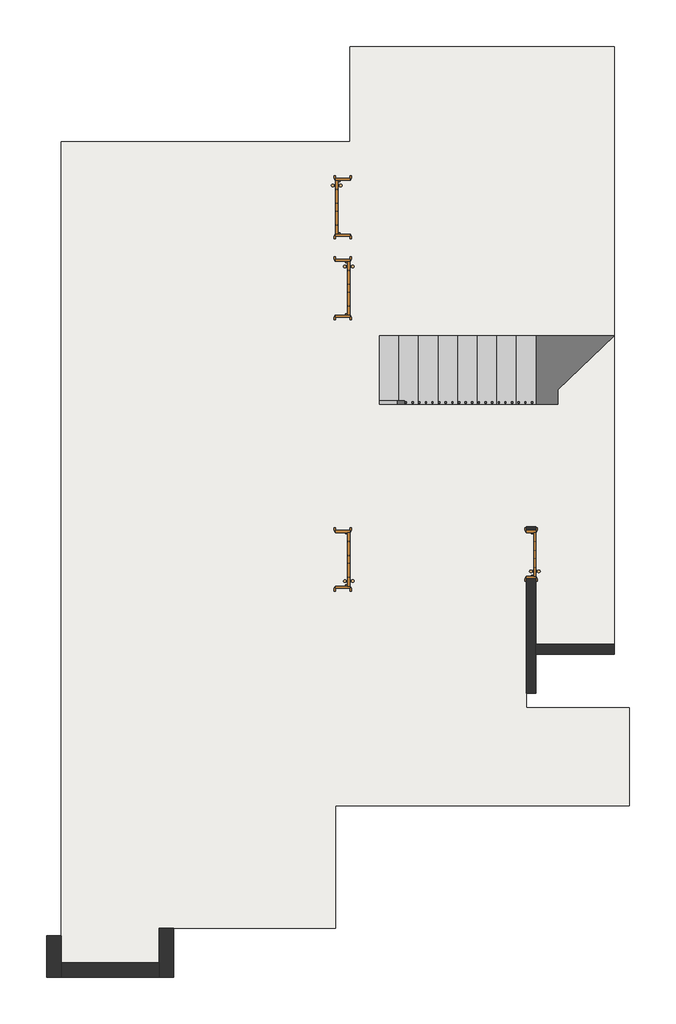
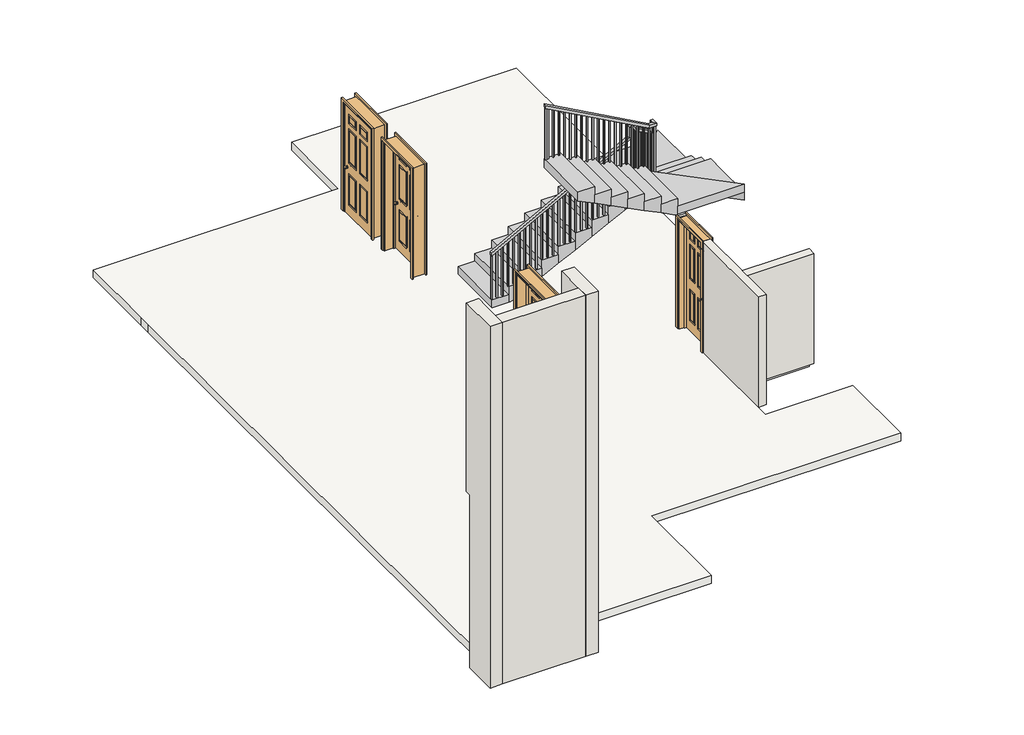
# One storey: 5 walls, 4 doors, 1 railing, 1 slab, 1 stair flight.
"""IFC4 building model written with IfcOpenShell, lengths in millimetres."""

from ifc_helpers import new_model, si_unit, frame, origin, place, context, project, spatial, polyline, outline, extrude, faceted_brep, transform, mapped, element, save
from components import intsgl_9_d1_c400c9dc, intsgl_9_d1_bc548916, intsgl_9_d2_a593ccd7

model = new_model("IFC4")

# Units and contexts
model_context = context("Model", 3, world=origin())
ifc_project = project(units=[si_unit("LENGTHUNIT", "METRE", prefix="MILLI")], contexts=[model_context])

# Site, building, storey
site = spatial("IfcSite", under=ifc_project)
building = spatial("IfcBuilding", under=site)
storey = spatial("IfcBuildingStorey", under=building, Elevation=600.0)

# Doors
placement = place(None, origin())
intsgl_9_d1_shape = intsgl_9_d1_c400c9dc(model_context)
element("IfcDoor", 1, ObjectType="IntSgl (9) : D1", at=placement, inside=storey, context=model_context, shape_type="MappedRepresentation", body=[
    mapped(intsgl_9_d1_shape, transform((-10030.1792561, 3948.2802318, 600.0), x_axis=(0.0, -1.0, 0.0), y_axis=(1.0, 0.0, 0.0), z_axis=(0.0, 0.0, 1.0))),
])
intsgl_9_d1_2_shape = intsgl_9_d1_bc548916(model_context)
element("IfcDoor", 2, ObjectType="IntSgl (9) : D1", at=placement, inside=storey, context=model_context, shape_type="MappedRepresentation", body=[
    mapped(intsgl_9_d1_2_shape, transform((-10030.1792561, 5188.2802318, 600.0), x_axis=(0.0, -1.0, 0.0), y_axis=(1.0, 0.0, 0.0), z_axis=(0.0, 0.0, 1.0))),
])
element("IfcDoor", 3, ObjectType="IntSgl (9) : D1", at=placement, inside=storey, context=model_context, shape_type="MappedRepresentation", body=[
    mapped(intsgl_9_d1_2_shape, transform((-10030.1792561, -201.7197682, 600.0), x_axis=(0.0, 1.0, 0.0), y_axis=(-1.0, 0.0, 0.0), z_axis=(0.0, 0.0, 1.0))),
])
intsgl_9_d2_shape = intsgl_9_d2_a593ccd7(model_context)
element("IfcDoor", 4, ObjectType="IntSgl (9) : D2", at=placement, inside=storey, context=model_context, shape_type="MappedRepresentation", body=[
    mapped(intsgl_9_d2_shape, transform((-7142.6792561, -126.7197682, 600.0), x_axis=(0.0, 1.0, 0.0), y_axis=(-1.0, 0.0, 0.0), z_axis=(0.0, 0.0, 1.0))),
])

# Railing
element("IfcRailing", 5, ObjectType="Handrail - Rectangular", at=placement, inside=storey, context=model_context, shape_type="SolidModel", body=[
    faceted_brep([(-9467.6792561, 2223.6802318, 1650.0), (-9467.6792561, 2223.6802318, 1593.1757094), (-9467.6792561, 2173.6802318, 1593.1757094), (-9467.6792561, 2173.6802318, 1650.0), (-6992.2792561, 2223.6802318, 2986.716), (-6942.2792561, 2223.6802318, 2956.8917094), (-6942.2792561, 2173.6802318, 2956.8917094), (-6992.2792561, 2173.6802318, 2986.716), (-6992.2792561, 2223.6802318, 3187.3), (-6942.2792561, 2223.6802318, 3137.3), (-6942.2792561, 2173.6802318, 3137.3), (-6992.2792561, 2173.6802318, 3187.3), (-6867.2792561, 2223.6802318, 3187.3), (-6867.2792561, 2223.6802318, 3137.3), (-6917.2792561, 2173.6802318, 3137.3), (-6917.2792561, 2173.6802318, 3187.3), (-6867.2792561, 2098.6802318, 3187.3), (-6867.2792561, 2086.8768329, 3137.3), (-6917.2792561, 2086.8768329, 3137.3), (-6917.2792561, 2098.6802318, 3187.3), (-6867.2792561, 1647.8802318, 3412.7), (-6867.2792561, 1597.8802318, 3381.7983006), (-6917.2792561, 1597.8802318, 3381.7983006), (-6917.2792561, 1647.8802318, 3412.7), (-6867.2792561, 1647.8802318, 3613.5947368), (-6867.2792561, 1597.8802318, 3563.5947368), (-6917.2792561, 1597.8802318, 3563.5947368), (-6917.2792561, 1647.8802318, 3613.5947368), (-6867.2792561, 1522.8802318, 3613.5947368), (-6867.2792561, 1522.8802318, 3563.5947368), (-6917.2792561, 1572.8802318, 3563.5947368), (-6917.2792561, 1572.8802318, 3613.5947368), (-6992.2792561, 1522.8802318, 3613.5947368), (-7005.1758911, 1522.8802318, 3563.5947368), (-7005.1758911, 1572.8802318, 3563.5947368), (-6992.2792561, 1572.8802318, 3613.5947368), (-8867.6792561, 1522.8802318, 4650.0), (-8867.6792561, 1572.8802318, 4650.0), (-8867.6792561, 1572.8802318, 4592.8729122), (-8867.6792561, 1522.8802318, 4592.8729122)], [[[0, 1, 2, 3]], [[1, 0, 4, 5]], [[2, 1, 5, 6]], [[3, 2, 6, 7]], [[0, 3, 7, 4]], [[5, 4, 8, 9]], [[6, 5, 9, 10]], [[7, 6, 10, 11]], [[4, 7, 11, 8]], [[9, 8, 12, 13]], [[10, 9, 13, 14]], [[11, 10, 14, 15]], [[8, 11, 15, 12]], [[13, 12, 16, 17]], [[14, 13, 17, 18]], [[15, 14, 18, 19]], [[12, 15, 19, 16]], [[17, 16, 20, 21]], [[18, 17, 21, 22]], [[19, 18, 22, 23]], [[16, 19, 23, 20]], [[21, 20, 24, 25]], [[22, 21, 25, 26]], [[23, 22, 26, 27]], [[20, 23, 27, 24]], [[25, 24, 28, 29]], [[26, 25, 29, 30]], [[27, 26, 30, 31]], [[24, 27, 31, 28]], [[29, 28, 32, 33]], [[30, 29, 33, 34]], [[31, 30, 34, 35]], [[28, 31, 35, 32]], [[36, 37, 38, 39]], [[33, 32, 36, 39]], [[34, 33, 39, 38]], [[35, 34, 38, 37]], [[32, 35, 37, 36]]]),
    extrude(outline(polyline([(3600.0, -8812.6792561), (4562.4781754, -8812.6792561), (4573.530807, -8832.6792561), (3600.0, -8832.6792561), (3600.0, -8812.6792561)])), frame((0.0, 1537.8802318, 0.0), z_axis=(0.0, 1.0, 0.0), x_axis=(0.0, 0.0, 1.0)), (0.0, 0.0, 1.0), 20.0),
    extrude(outline(polyline([(3600.0, -8711.0792561), (4506.330807, -8711.0792561), (4517.3834386, -8731.0792561), (3600.0, -8731.0792561), (3600.0, -8711.0792561)])), frame((0.0, 1537.8802318, 0.0), z_axis=(0.0, 1.0, 0.0), x_axis=(0.0, 0.0, 1.0)), (0.0, 0.0, 1.0), 20.0),
    extrude(outline(polyline([(3600.0, -8609.4792561), (4450.1834386, -8609.4792561), (4461.2360701, -8629.4792561), (3600.0, -8629.4792561), (3600.0, -8609.4792561)])), frame((0.0, 1537.8802318, 0.0), z_axis=(0.0, 1.0, 0.0), x_axis=(0.0, 0.0, 1.0)), (0.0, 0.0, 1.0), 20.0),
    extrude(outline(polyline([(3450.0, -8507.8792561), (4394.0360701, -8507.8792561), (4405.0887017, -8527.8792561), (3450.0, -8527.8792561), (3450.0, -8507.8792561)])), frame((0.0, 1537.8802318, 0.0), z_axis=(0.0, 1.0, 0.0), x_axis=(0.0, 0.0, 1.0)), (0.0, 0.0, 1.0), 20.0),
    extrude(outline(polyline([(3450.0, -8406.2792561), (4337.8887017, -8406.2792561), (4348.9413333, -8426.2792561), (3450.0, -8426.2792561), (3450.0, -8406.2792561)])), frame((0.0, 1537.8802318, 0.0), z_axis=(0.0, 1.0, 0.0), x_axis=(0.0, 0.0, 1.0)), (0.0, 0.0, 1.0), 20.0),
    extrude(outline(polyline([(3450.0, -8304.6792561), (4281.7413333, -8304.6792561), (4292.7939649, -8324.6792561), (3450.0, -8324.6792561), (3450.0, -8304.6792561)])), frame((0.0, 1537.8802318, 0.0), z_axis=(0.0, 1.0, 0.0), x_axis=(0.0, 0.0, 1.0)), (0.0, 0.0, 1.0), 20.0),
    extrude(outline(polyline([(3300.0, -8203.0792561), (4225.5939649, -8203.0792561), (4236.6465965, -8223.0792561), (3300.0, -8223.0792561), (3300.0, -8203.0792561)])), frame((0.0, 1537.8802318, 0.0), z_axis=(0.0, 1.0, 0.0), x_axis=(0.0, 0.0, 1.0)), (0.0, 0.0, 1.0), 20.0),
    extrude(outline(polyline([(3300.0, -8101.4792561), (4169.4465965, -8101.4792561), (4180.499228, -8121.4792561), (3300.0, -8121.4792561), (3300.0, -8101.4792561)])), frame((0.0, 1537.8802318, 0.0), z_axis=(0.0, 1.0, 0.0), x_axis=(0.0, 0.0, 1.0)), (0.0, 0.0, 1.0), 20.0),
    extrude(outline(polyline([(3300.0, -7999.8792561), (4113.299228, -7999.8792561), (4124.3518596, -8019.8792561), (3300.0, -8019.8792561), (3300.0, -7999.8792561)])), frame((0.0, 1537.8802318, 0.0), z_axis=(0.0, 1.0, 0.0), x_axis=(0.0, 0.0, 1.0)), (0.0, 0.0, 1.0), 20.0),
    extrude(outline(polyline([(3150.0, -7898.2792561), (4057.1518596, -7898.2792561), (4068.2044912, -7918.2792561), (3150.0, -7918.2792561), (3150.0, -7898.2792561)])), frame((0.0, 1537.8802318, 0.0), z_axis=(0.0, 1.0, 0.0), x_axis=(0.0, 0.0, 1.0)), (0.0, 0.0, 1.0), 20.0),
    extrude(outline(polyline([(3150.0, -7796.6792561), (4001.0044912, -7796.6792561), (4012.0571228, -7816.6792561), (3150.0, -7816.6792561), (3150.0, -7796.6792561)])), frame((0.0, 1537.8802318, 0.0), z_axis=(0.0, 1.0, 0.0), x_axis=(0.0, 0.0, 1.0)), (0.0, 0.0, 1.0), 20.0),
    extrude(outline(polyline([(3150.0, -7695.0792561), (3944.8571228, -7695.0792561), (3955.9097544, -7715.0792561), (3150.0, -7715.0792561), (3150.0, -7695.0792561)])), frame((0.0, 1537.8802318, 0.0), z_axis=(0.0, 1.0, 0.0), x_axis=(0.0, 0.0, 1.0)), (0.0, 0.0, 1.0), 20.0),
    extrude(outline(polyline([(3000.0, -7593.4792561), (3888.7097544, -7593.4792561), (3899.7623859, -7613.4792561), (3000.0, -7613.4792561), (3000.0, -7593.4792561)])), frame((0.0, 1537.8802318, 0.0), z_axis=(0.0, 1.0, 0.0), x_axis=(0.0, 0.0, 1.0)), (0.0, 0.0, 1.0), 20.0),
    extrude(outline(polyline([(3000.0, -7491.8792561), (3832.5623859, -7491.8792561), (3843.6150175, -7511.8792561), (3000.0, -7511.8792561), (3000.0, -7491.8792561)])), frame((0.0, 1537.8802318, 0.0), z_axis=(0.0, 1.0, 0.0), x_axis=(0.0, 0.0, 1.0)), (0.0, 0.0, 1.0), 20.0),
    extrude(outline(polyline([(3000.0, -7390.2792561), (3776.4150175, -7390.2792561), (3787.4676491, -7410.2792561), (3000.0, -7410.2792561), (3000.0, -7390.2792561)])), frame((0.0, 1537.8802318, 0.0), z_axis=(0.0, 1.0, 0.0), x_axis=(0.0, 0.0, 1.0)), (0.0, 0.0, 1.0), 20.0),
    extrude(outline(polyline([(2850.0, -7288.6792561), (3720.2676491, -7288.6792561), (3731.3202807, -7308.6792561), (2850.0, -7308.6792561), (2850.0, -7288.6792561)])), frame((0.0, 1537.8802318, 0.0), z_axis=(0.0, 1.0, 0.0), x_axis=(0.0, 0.0, 1.0)), (0.0, 0.0, 1.0), 20.0),
    extrude(outline(polyline([(2850.0, -7187.0792561), (3664.1202807, -7187.0792561), (3675.1729122, -7207.0792561), (2850.0, -7207.0792561), (2850.0, -7187.0792561)])), frame((0.0, 1537.8802318, 0.0), z_axis=(0.0, 1.0, 0.0), x_axis=(0.0, 0.0, 1.0)), (0.0, 0.0, 1.0), 20.0),
    extrude(outline(polyline([(2850.0, -7085.4792561), (3607.9729122, -7085.4792561), (3619.0255438, -7105.4792561), (2850.0, -7105.4792561), (2850.0, -7085.4792561)])), frame((0.0, 1537.8802318, 0.0), z_axis=(0.0, 1.0, 0.0), x_axis=(0.0, 0.0, 1.0)), (0.0, 0.0, 1.0), 20.0),
    extrude(outline(polyline([(2700.0, -6983.8792561), (3551.8255438, -6983.8792561), (3562.8781754, -7003.8792561), (2700.0, -7003.8792561), (2700.0, -6983.8792561)])), frame((0.0, 1537.8802318, 0.0), z_axis=(0.0, 1.0, 0.0), x_axis=(0.0, 0.0, 1.0)), (0.0, 0.0, 1.0), 20.0),
    extrude(outline(polyline([(-6902.2792561, 1599.0802318), (-6882.2792561, 1599.0802318), (-6882.2792561, 1579.0802318), (-6902.2792561, 1579.0802318), (-6902.2792561, 1599.0802318)])), frame((0.0, 0.0, 2400.0), z_axis=(0.0, 0.0, 1.0), x_axis=(1.0, 0.0, 0.0)), (0.0, 0.0, 1.0), 1163.5947368),
    extrude(outline(polyline([(1700.6802318, 3330.3983006), (1700.6802318, 2400.0), (1680.6802318, 2400.0), (1680.6802318, 3340.3983006), (1700.6802318, 3330.3983006)])), frame((-6902.2792561, 0.0, 0.0), z_axis=(1.0, 0.0, 0.0), x_axis=(0.0, 1.0, 0.0)), (0.0, 0.0, 1.0), 20.0),
    extrude(outline(polyline([(1802.2802318, 3279.5983006), (1802.2802318, 2400.0), (1782.2802318, 2400.0), (1782.2802318, 3289.5983006), (1802.2802318, 3279.5983006)])), frame((-6902.2792561, 0.0, 0.0), z_axis=(1.0, 0.0, 0.0), x_axis=(0.0, 1.0, 0.0)), (0.0, 0.0, 1.0), 20.0),
    extrude(outline(polyline([(1903.8802318, 3228.7983006), (1903.8802318, 2250.0), (1883.8802318, 2250.0), (1883.8802318, 3238.7983006), (1903.8802318, 3228.7983006)])), frame((-6902.2792561, 0.0, 0.0), z_axis=(1.0, 0.0, 0.0), x_axis=(0.0, 1.0, 0.0)), (0.0, 0.0, 1.0), 20.0),
    extrude(outline(polyline([(2005.4802318, 3177.9983006), (2005.4802318, 2250.0), (1985.4802318, 2250.0), (1985.4802318, 3187.9983006), (2005.4802318, 3177.9983006)])), frame((-6902.2792561, 0.0, 0.0), z_axis=(1.0, 0.0, 0.0), x_axis=(0.0, 1.0, 0.0)), (0.0, 0.0, 1.0), 20.0),
    extrude(outline(polyline([(2107.0802318, 3127.1983006), (2107.0802318, 2250.0), (2087.0802318, 2250.0), (2087.0802318, 3137.1983006), (2107.0802318, 3127.1983006)])), frame((-6902.2792561, 0.0, 0.0), z_axis=(1.0, 0.0, 0.0), x_axis=(0.0, 1.0, 0.0)), (0.0, 0.0, 1.0), 20.0),
    extrude(outline(polyline([(-6937.6792561, 2188.6802318), (-6937.6792561, 2208.6802318), (-6917.6792561, 2208.6802318), (-6917.6792561, 2188.6802318), (-6937.6792561, 2188.6802318)])), frame((0.0, 0.0, 2100.0), z_axis=(0.0, 0.0, 1.0), x_axis=(1.0, 0.0, 0.0)), (0.0, 0.0, 1.0), 1037.3),
    extrude(outline(polyline([(2904.5117094, -7039.2792561), (1950.0, -7039.2792561), (1950.0, -7019.2792561), (2915.3117094, -7019.2792561), (2904.5117094, -7039.2792561)])), frame((0.0, 2188.6802318, 0.0), z_axis=(0.0, 1.0, 0.0), x_axis=(0.0, 0.0, 1.0)), (0.0, 0.0, 1.0), 20.0),
    extrude(outline(polyline([(2849.6477094, -7140.8792561), (1800.0, -7140.8792561), (1800.0, -7120.8792561), (2860.4477094, -7120.8792561), (2849.6477094, -7140.8792561)])), frame((0.0, 2188.6802318, 0.0), z_axis=(0.0, 1.0, 0.0), x_axis=(0.0, 0.0, 1.0)), (0.0, 0.0, 1.0), 20.0),
    extrude(outline(polyline([(2794.7837094, -7242.4792561), (1800.0, -7242.4792561), (1800.0, -7222.4792561), (2805.5837094, -7222.4792561), (2794.7837094, -7242.4792561)])), frame((0.0, 2188.6802318, 0.0), z_axis=(0.0, 1.0, 0.0), x_axis=(0.0, 0.0, 1.0)), (0.0, 0.0, 1.0), 20.0),
    extrude(outline(polyline([(2739.9197094, -7344.0792561), (1800.0, -7344.0792561), (1800.0, -7324.0792561), (2750.7197094, -7324.0792561), (2739.9197094, -7344.0792561)])), frame((0.0, 2188.6802318, 0.0), z_axis=(0.0, 1.0, 0.0), x_axis=(0.0, 0.0, 1.0)), (0.0, 0.0, 1.0), 20.0),
    extrude(outline(polyline([(2685.0557094, -7445.6792561), (1650.0, -7445.6792561), (1650.0, -7425.6792561), (2695.8557094, -7425.6792561), (2685.0557094, -7445.6792561)])), frame((0.0, 2188.6802318, 0.0), z_axis=(0.0, 1.0, 0.0), x_axis=(0.0, 0.0, 1.0)), (0.0, 0.0, 1.0), 20.0),
    extrude(outline(polyline([(2630.1917094, -7547.2792561), (1650.0, -7547.2792561), (1650.0, -7527.2792561), (2640.9917094, -7527.2792561), (2630.1917094, -7547.2792561)])), frame((0.0, 2188.6802318, 0.0), z_axis=(0.0, 1.0, 0.0), x_axis=(0.0, 0.0, 1.0)), (0.0, 0.0, 1.0), 20.0),
    extrude(outline(polyline([(2575.3277094, -7648.8792561), (1650.0, -7648.8792561), (1650.0, -7628.8792561), (2586.1277094, -7628.8792561), (2575.3277094, -7648.8792561)])), frame((0.0, 2188.6802318, 0.0), z_axis=(0.0, 1.0, 0.0), x_axis=(0.0, 0.0, 1.0)), (0.0, 0.0, 1.0), 20.0),
    extrude(outline(polyline([(2520.4637094, -7750.4792561), (1500.0, -7750.4792561), (1500.0, -7730.4792561), (2531.2637094, -7730.4792561), (2520.4637094, -7750.4792561)])), frame((0.0, 2188.6802318, 0.0), z_axis=(0.0, 1.0, 0.0), x_axis=(0.0, 0.0, 1.0)), (0.0, 0.0, 1.0), 20.0),
    extrude(outline(polyline([(2465.5997094, -7852.0792561), (1500.0, -7852.0792561), (1500.0, -7832.0792561), (2476.3997094, -7832.0792561), (2465.5997094, -7852.0792561)])), frame((0.0, 2188.6802318, 0.0), z_axis=(0.0, 1.0, 0.0), x_axis=(0.0, 0.0, 1.0)), (0.0, 0.0, 1.0), 20.0),
    extrude(outline(polyline([(2410.7357094, -7953.6792561), (1500.0, -7953.6792561), (1500.0, -7933.6792561), (2421.5357094, -7933.6792561), (2410.7357094, -7953.6792561)])), frame((0.0, 2188.6802318, 0.0), z_axis=(0.0, 1.0, 0.0), x_axis=(0.0, 0.0, 1.0)), (0.0, 0.0, 1.0), 20.0),
    extrude(outline(polyline([(2355.8717094, -8055.2792561), (1350.0, -8055.2792561), (1350.0, -8035.2792561), (2366.6717094, -8035.2792561), (2355.8717094, -8055.2792561)])), frame((0.0, 2188.6802318, 0.0), z_axis=(0.0, 1.0, 0.0), x_axis=(0.0, 0.0, 1.0)), (0.0, 0.0, 1.0), 20.0),
    extrude(outline(polyline([(2301.0077094, -8156.8792561), (1350.0, -8156.8792561), (1350.0, -8136.8792561), (2311.8077094, -8136.8792561), (2301.0077094, -8156.8792561)])), frame((0.0, 2188.6802318, 0.0), z_axis=(0.0, 1.0, 0.0), x_axis=(0.0, 0.0, 1.0)), (0.0, 0.0, 1.0), 20.0),
    extrude(outline(polyline([(2246.1437094, -8258.4792561), (1350.0, -8258.4792561), (1350.0, -8238.4792561), (2256.9437094, -8238.4792561), (2246.1437094, -8258.4792561)])), frame((0.0, 2188.6802318, 0.0), z_axis=(0.0, 1.0, 0.0), x_axis=(0.0, 0.0, 1.0)), (0.0, 0.0, 1.0), 20.0),
    extrude(outline(polyline([(2191.2797094, -8360.0792561), (1200.0, -8360.0792561), (1200.0, -8340.0792561), (2202.0797094, -8340.0792561), (2191.2797094, -8360.0792561)])), frame((0.0, 2188.6802318, 0.0), z_axis=(0.0, 1.0, 0.0), x_axis=(0.0, 0.0, 1.0)), (0.0, 0.0, 1.0), 20.0),
    extrude(outline(polyline([(2136.4157094, -8461.6792561), (1200.0, -8461.6792561), (1200.0, -8441.6792561), (2147.2157094, -8441.6792561), (2136.4157094, -8461.6792561)])), frame((0.0, 2188.6802318, 0.0), z_axis=(0.0, 1.0, 0.0), x_axis=(0.0, 0.0, 1.0)), (0.0, 0.0, 1.0), 20.0),
    extrude(outline(polyline([(2081.5517094, -8563.2792561), (1200.0, -8563.2792561), (1200.0, -8543.2792561), (2092.3517094, -8543.2792561), (2081.5517094, -8563.2792561)])), frame((0.0, 2188.6802318, 0.0), z_axis=(0.0, 1.0, 0.0), x_axis=(0.0, 0.0, 1.0)), (0.0, 0.0, 1.0), 20.0),
    extrude(outline(polyline([(2026.6877094, -8664.8792561), (1050.0, -8664.8792561), (1050.0, -8644.8792561), (2037.4877094, -8644.8792561), (2026.6877094, -8664.8792561)])), frame((0.0, 2188.6802318, 0.0), z_axis=(0.0, 1.0, 0.0), x_axis=(0.0, 0.0, 1.0)), (0.0, 0.0, 1.0), 20.0),
    extrude(outline(polyline([(1971.8237094, -8766.4792561), (1050.0, -8766.4792561), (1050.0, -8746.4792561), (1982.6237094, -8746.4792561), (1971.8237094, -8766.4792561)])), frame((0.0, 2188.6802318, 0.0), z_axis=(0.0, 1.0, 0.0), x_axis=(0.0, 0.0, 1.0)), (0.0, 0.0, 1.0), 20.0),
    extrude(outline(polyline([(1916.9597094, -8868.0792561), (1050.0, -8868.0792561), (1050.0, -8848.0792561), (1927.7597094, -8848.0792561), (1916.9597094, -8868.0792561)])), frame((0.0, 2188.6802318, 0.0), z_axis=(0.0, 1.0, 0.0), x_axis=(0.0, 0.0, 1.0)), (0.0, 0.0, 1.0), 20.0),
    extrude(outline(polyline([(1862.0957094, -8969.6792561), (900.0, -8969.6792561), (900.0, -8949.6792561), (1872.8957094, -8949.6792561), (1862.0957094, -8969.6792561)])), frame((0.0, 2188.6802318, 0.0), z_axis=(0.0, 1.0, 0.0), x_axis=(0.0, 0.0, 1.0)), (0.0, 0.0, 1.0), 20.0),
    extrude(outline(polyline([(1807.2317094, -9071.2792561), (900.0, -9071.2792561), (900.0, -9051.2792561), (1818.0317094, -9051.2792561), (1807.2317094, -9071.2792561)])), frame((0.0, 2188.6802318, 0.0), z_axis=(0.0, 1.0, 0.0), x_axis=(0.0, 0.0, 1.0)), (0.0, 0.0, 1.0), 20.0),
    extrude(outline(polyline([(1752.3677094, -9172.8792561), (900.0, -9172.8792561), (900.0, -9152.8792561), (1763.1677094, -9152.8792561), (1752.3677094, -9172.8792561)])), frame((0.0, 2188.6802318, 0.0), z_axis=(0.0, 1.0, 0.0), x_axis=(0.0, 0.0, 1.0)), (0.0, 0.0, 1.0), 20.0),
    extrude(outline(polyline([(1697.5037094, -9274.4792561), (750.0, -9274.4792561), (750.0, -9254.4792561), (1708.3037094, -9254.4792561), (1697.5037094, -9274.4792561)])), frame((0.0, 2188.6802318, 0.0), z_axis=(0.0, 1.0, 0.0), x_axis=(0.0, 0.0, 1.0)), (0.0, 0.0, 1.0), 20.0),
    extrude(outline(polyline([(1642.6397094, -9376.0792561), (750.0, -9376.0792561), (750.0, -9356.0792561), (1653.4397094, -9356.0792561), (1642.6397094, -9376.0792561)])), frame((0.0, 2188.6802318, 0.0), z_axis=(0.0, 1.0, 0.0), x_axis=(0.0, 0.0, 1.0)), (0.0, 0.0, 1.0), 20.0),
    extrude(outline(polyline([(-6902.2792561, 1557.8802318), (-6882.2792561, 1557.8802318), (-6882.2792561, 1537.8802318), (-6902.2792561, 1537.8802318), (-6902.2792561, 1557.8802318)])), frame((0.0, 0.0, 2550.0), z_axis=(0.0, 0.0, 1.0), x_axis=(1.0, 0.0, 0.0)), (0.0, 0.0, 1.0), 1013.5947368),
    extrude(outline(polyline([(-6902.2792561, 2188.6802318), (-6902.2792561, 2208.6802318), (-6882.2792561, 2208.6802318), (-6882.2792561, 2188.6802318), (-6902.2792561, 2188.6802318)])), frame((0.0, 0.0, 2100.0), z_axis=(0.0, 0.0, 1.0), x_axis=(1.0, 0.0, 0.0)), (0.0, 0.0, 1.0), 1037.3),
    extrude(outline(polyline([(3600.0, -8848.1792561), (4582.0965965, -8848.1792561), (4593.149228, -8868.1792561), (3600.0, -8868.1792561), (3600.0, -8848.1792561)])), frame((0.0, 1537.8802318, 0.0), z_axis=(0.0, 1.0, 0.0), x_axis=(0.0, 0.0, 1.0)), (0.0, 0.0, 1.0), 20.0),
    extrude(outline(polyline([(1592.9057094, -9468.1792561), (750.0, -9468.1792561), (750.0, -9448.1792561), (1603.7057094, -9448.1792561), (1592.9057094, -9468.1792561)])), frame((0.0, 2188.6802318, 0.0), z_axis=(0.0, 1.0, 0.0), x_axis=(0.0, 0.0, 1.0)), (0.0, 0.0, 1.0), 20.0),
])

# Slab
element("IfcSlab", 6, ObjectType="01-floor", at=placement, inside=storey, context=model_context, shape_type="SweptSolid", body=[
    extrude(outline(polyline([(-9917.6792561, 7648.2802318), (-5867.6792561, 7648.2802318), (-5867.6792561, -1501.7197682), (-7217.6792561, -1501.7197682), (-7217.6792561, -2051.7197682), (-7217.6792561, -2476.7197682), (-5642.6792561, -2476.7197682), (-5642.6792561, -3976.7197682), (-10142.6792561, -3976.7197682), (-10142.6792561, -5851.7197682), (-12842.6792561, -5851.7197682), (-12842.6792561, -6376.7197682), (-14342.6792561, -6376.7197682), (-14342.6792561, 4463.2802318), (-14342.6792561, 4688.2802318), (-14342.6792561, 6188.2802318), (-9917.6792561, 6188.2802318), (-9917.6792561, 7648.2802318)])), frame((0.0, 0.0, 450.0), z_axis=(0.0, 0.0, 1.0), x_axis=(1.0, 0.0, 0.0)), (0.0, 0.0, 1.0), 150.0),
])

# Stair flight
element("IfcStairFlight", 7, ObjectType="M_Monolithic Run", at=placement, inside=storey, context=model_context, shape_type="Brep", body=[
    faceted_brep([(-9167.6792561, 3223.2802318, 750.0), (-9467.6792561, 3223.2802318, 750.0), (-9467.6792561, 2173.2802318, 750.0), (-9167.6792561, 2173.2802318, 750.0), (-9167.6792561, 3223.2802318, 600.0), (-9467.6792561, 3223.2802318, 600.0), (-9467.6792561, 2173.2802318, 600.0), (-9167.6792561, 2173.2802318, 600.0), (-8867.6792561, 3223.2802318, 900.0), (-9167.6792561, 3223.2802318, 900.0), (-9167.6792561, 2173.2802318, 900.0), (-8867.6792561, 2173.2802318, 900.0), (-8867.6792561, 3223.2802318, 732.2949017), (-9132.2690595, 3223.2802318, 600.0), (-9132.2690595, 2173.2802318, 600.0), (-8867.6792561, 2173.2802318, 732.2949017), (-8567.6792561, 3223.2802318, 1050.0), (-8867.6792561, 3223.2802318, 1050.0), (-8867.6792561, 2173.2802318, 1050.0), (-8567.6792561, 2173.2802318, 1050.0), (-8567.6792561, 3223.2802318, 882.2949017), (-8567.6792561, 2173.2802318, 882.2949017), (-8267.6792561, 3223.2802318, 1200.0), (-8567.6792561, 3223.2802318, 1200.0), (-8567.6792561, 2173.2802318, 1200.0), (-8267.6792561, 2173.2802318, 1200.0), (-8267.6792561, 3223.2802318, 1032.2949017), (-8267.6792561, 2173.2802318, 1032.2949017), (-7967.6792561, 3223.2802318, 1350.0), (-8267.6792561, 3223.2802318, 1350.0), (-8267.6792561, 2173.2802318, 1350.0), (-7967.6792561, 2173.2802318, 1350.0), (-7967.6792561, 3223.2802318, 1182.2949017), (-7967.6792561, 2173.2802318, 1182.2949017), (-7667.6792561, 3223.2802318, 1500.0), (-7967.6792561, 3223.2802318, 1500.0), (-7967.6792561, 2173.2802318, 1500.0), (-7667.6792561, 2173.2802318, 1500.0), (-7667.6792561, 3223.2802318, 1332.2949017), (-7667.6792561, 2173.2802318, 1332.2949017), (-7367.6792561, 3223.2802318, 1650.0), (-7667.6792561, 3223.2802318, 1650.0), (-7667.6792561, 2173.2802318, 1650.0), (-7367.6792561, 2173.2802318, 1650.0), (-7367.6792561, 3223.2802318, 1482.2949017), (-7367.6792561, 2173.2802318, 1482.2949017), (-7067.6792561, 3223.2802318, 1800.0), (-7367.6792561, 3223.2802318, 1800.0), (-7367.6792561, 2173.2802318, 1800.0), (-7067.6792561, 2173.2802318, 1800.0), (-7067.6792561, 3223.2802318, 1632.2949017), (-7067.6792561, 2173.2802318, 1632.2949017), (-7067.6792561, 3223.2802318, 1950.0), (-7067.6792561, 2173.2802318, 1950.0), (-6967.6792561, 2173.2802318, 1950.0), (-6732.2690595, 2397.9899649, 1950.0), (-5867.6792561, 3223.2802318, 1950.0), (-6732.2690595, 3223.2802318, 1950.0), (-5867.6792561, 3223.2802318, 1800.0), (-6732.2690595, 3223.2802318, 1800.0), (-6967.6792561, 2173.2802318, 1682.2949017), (-5867.6792561, 2173.2802318, 2100.0), (-5867.6792561, 3223.2802318, 2100.0), (-6967.6792561, 2173.2802318, 2100.0), (-6917.6792561, 2173.2802318, 2100.0), (-5867.6792561, 2173.2802318, 1950.0), (-6732.2690595, 2173.2802318, 1800.0), (-6732.2690595, 2173.2802318, 1950.0), (-6917.6792561, 2173.2802318, 1950.0), (-5867.6792561, 2173.2802318, 2250.0), (-6917.6792561, 2173.2802318, 2250.0), (-6917.6792561, 2137.8700351, 2250.0), (-6917.6792561, 1873.2802318, 2250.0), (-5867.6792561, 1873.2802318, 2250.0), (-5867.6792561, 2137.8700351, 2250.0), (-5867.6792561, 1873.2802318, 2082.2949017), (-5867.6792561, 2137.8700351, 1950.0), (-6917.6792561, 2137.8700351, 1950.0), (-6917.6792561, 1873.2802318, 2082.2949017), (-5867.6792561, 1573.2802318, 2400.0), (-5867.6792561, 1873.2802318, 2400.0), (-6917.6792561, 1873.2802318, 2400.0), (-6917.6792561, 1573.2802318, 2400.0), (-5867.6792561, 1573.2802318, 2232.2949017), (-6917.6792561, 1237.8700351, 2400.0), (-6917.6792561, 1237.8700351, 2550.0), (-6917.6792561, 1525.552959, 2550.0), (-6917.6792561, 1573.2802318, 2550.0), (-5867.6792561, 1573.2802318, 2550.0), (-6616.2971454, 1237.8700351, 2550.0), (-5867.6792561, 523.2802318, 2550.0), (-5867.6792561, 1237.8700351, 2550.0), (-5867.6792561, 523.2802318, 2400.0), (-5867.6792561, 1237.8700351, 2400.0), (-7067.6792561, 523.2802318, 2700.0), (-5867.6792561, 523.2802318, 2700.0), (-6917.6792561, 1525.552959, 2700.0), (-6967.6792561, 1573.2802318, 2700.0), (-7067.6792561, 1573.2802318, 2700.0), (-7067.6792561, 523.2802318, 2550.0), (-6967.6792561, 1573.2802318, 2550.0), (-7067.6792561, 1573.2802318, 2550.0), (-6732.2690595, 2397.9899649, 1800.0), (-6732.2690595, 2397.9899649, 1950.0), (-6616.2971454, 1237.8700351, 2400.0), (-6616.2971454, 1237.8700351, 2550.0), (-7103.0894527, 523.2802318, 2550.0), (-7103.0894527, 1573.2802318, 2550.0), (-7067.6792561, 523.2802318, 2850.0), (-7067.6792561, 1573.2802318, 2850.0), (-7103.0894527, 1573.2802318, 2850.0), (-7367.6792561, 1573.2802318, 2850.0), (-7367.6792561, 523.2802318, 2850.0), (-7103.0894527, 523.2802318, 2850.0), (-7367.6792561, 523.2802318, 2682.2949017), (-7367.6792561, 1573.2802318, 2682.2949017), (-7667.6792561, 523.2802318, 3000.0), (-7367.6792561, 523.2802318, 3000.0), (-7367.6792561, 1573.2802318, 3000.0), (-7667.6792561, 1573.2802318, 3000.0), (-7667.6792561, 523.2802318, 2832.2949017), (-7667.6792561, 1573.2802318, 2832.2949017), (-7967.6792561, 523.2802318, 3150.0), (-7667.6792561, 523.2802318, 3150.0), (-7667.6792561, 1573.2802318, 3150.0), (-7967.6792561, 1573.2802318, 3150.0), (-7967.6792561, 523.2802318, 2982.2949017), (-7967.6792561, 1573.2802318, 2982.2949017), (-8267.6792561, 523.2802318, 3300.0), (-7967.6792561, 523.2802318, 3300.0), (-7967.6792561, 1573.2802318, 3300.0), (-8267.6792561, 1573.2802318, 3300.0), (-8267.6792561, 523.2802318, 3132.2949017), (-8267.6792561, 1573.2802318, 3132.2949017), (-8567.6792561, 523.2802318, 3450.0), (-8267.6792561, 523.2802318, 3450.0), (-8267.6792561, 1573.2802318, 3450.0), (-8567.6792561, 1573.2802318, 3450.0), (-8567.6792561, 523.2802318, 3282.2949017), (-8567.6792561, 1573.2802318, 3282.2949017), (-8867.6792561, 523.2802318, 3600.0), (-8567.6792561, 523.2802318, 3600.0), (-8567.6792561, 1573.2802318, 3600.0), (-8867.6792561, 1573.2802318, 3600.0), (-8867.6792561, 523.2802318, 3432.2949017), (-8867.6792561, 1573.2802318, 3432.2949017)], [[[0, 1, 2, 3]], [[1, 0, 4, 5]], [[2, 1, 5, 6]], [[3, 2, 6, 7]], [[8, 9, 10, 11]], [[4, 0, 9, 8, 12, 13]], [[0, 3, 10, 9]], [[3, 7, 14, 15, 11, 10]], [[16, 17, 18, 19]], [[17, 16, 20, 12, 8]], [[8, 11, 18, 17]], [[19, 18, 11, 15, 21]], [[22, 23, 24, 25]], [[23, 22, 26, 20, 16]], [[16, 19, 24, 23]], [[25, 24, 19, 21, 27]], [[28, 29, 30, 31]], [[29, 28, 32, 26, 22]], [[22, 25, 30, 29]], [[31, 30, 25, 27, 33]], [[34, 35, 36, 37]], [[35, 34, 38, 32, 28]], [[28, 31, 36, 35]], [[37, 36, 31, 33, 39]], [[40, 41, 42, 43]], [[41, 40, 44, 38, 34]], [[34, 37, 42, 41]], [[43, 42, 37, 39, 45]], [[46, 47, 48, 49]], [[47, 46, 50, 44, 40]], [[40, 43, 48, 47]], [[49, 48, 43, 45, 51]], [[52, 53, 54, 55, 56, 57]], [[46, 52, 57, 56, 58, 59, 50]], [[46, 49, 53, 52]], [[54, 53, 49, 51, 60]], [[61, 62, 63, 64]], [[62, 61, 65, 56]], [[63, 62, 56, 55, 54]], [[64, 63, 54, 60, 66, 67, 68]], [[69, 70, 71, 72, 73, 74]], [[61, 69, 74, 73, 75, 76, 65]], [[61, 64, 70, 69]], [[70, 64, 68, 77, 78, 72, 71]], [[79, 80, 81, 82]], [[80, 79, 83, 75, 73]], [[73, 72, 81, 80]], [[82, 81, 72, 78, 84, 85, 86, 87]], [[88, 87, 86, 89, 90, 91]], [[79, 88, 91, 90, 92, 93, 83]], [[79, 82, 87, 88]], [[94, 95, 96, 97, 98]], [[95, 94, 99, 90]], [[95, 90, 89, 86, 100, 97, 96]], [[98, 97, 100, 101]], [[5, 4, 13, 14, 7, 6]], [[102, 66, 60, 51, 45, 39, 33, 27, 21, 15, 14, 13, 12, 20, 26, 32, 38, 44, 50, 59]], [[66, 102, 103, 67]], [[58, 102, 59]], [[102, 58, 56, 103]], [[67, 103, 56, 65, 76, 77, 68]], [[77, 76, 75, 83, 93, 104, 84, 78]], [[84, 104, 105, 85]], [[92, 104, 93]], [[104, 92, 90, 105]], [[85, 105, 90, 99, 106, 107, 101, 100, 86]], [[108, 109, 110, 111, 112, 113]], [[94, 108, 113, 112, 114, 106, 99]], [[94, 98, 109, 108]], [[109, 98, 101, 107, 115, 111, 110]], [[116, 117, 118, 119]], [[117, 116, 120, 114, 112]], [[112, 111, 118, 117]], [[119, 118, 111, 115, 121]], [[122, 123, 124, 125]], [[123, 122, 126, 120, 116]], [[116, 119, 124, 123]], [[125, 124, 119, 121, 127]], [[128, 129, 130, 131]], [[129, 128, 132, 126, 122]], [[122, 125, 130, 129]], [[131, 130, 125, 127, 133]], [[134, 135, 136, 137]], [[135, 134, 138, 132, 128]], [[128, 131, 136, 135]], [[137, 136, 131, 133, 139]], [[140, 141, 142, 143]], [[141, 140, 144, 138, 134]], [[134, 137, 142, 141]], [[143, 142, 137, 139, 145]], [[140, 143, 145, 144]], [[107, 106, 114, 120, 126, 132, 138, 144, 145, 139, 133, 127, 121, 115]]]),
])

# Walls
element("IfcWall", 8, ObjectType="02-150 WALL", at=placement, inside=storey, context=model_context, shape_type="Brep", body=[
    faceted_brep([(-7217.6792561, -2251.7197682, 600.0), (-7217.6792561, -2251.7197682, 2700.0), (-7217.6792561, -501.7197682, 2700.0), (-7217.6792561, -501.7197682, 600.0), (-7067.6792561, -2251.7197682, 2700.0), (-7067.6792561, -2251.7197682, 600.0), (-7067.6792561, -1651.7197682, 600.0), (-7067.6792561, -1501.7197682, 600.0), (-7067.6792561, -501.7197682, 600.0), (-7067.6792561, -501.7197682, 2700.0), (-7067.6792561, -1501.7197682, 2700.0), (-7067.6792561, -1651.7197682, 2700.0)], [[[0, 1, 2, 3]], [[4, 5, 6, 7, 8, 9, 10, 11]], [[5, 0, 3, 8, 7, 6]], [[1, 4, 11, 10, 9, 2]], [[1, 0, 5, 4]], [[3, 2, 9, 8]]]),
    faceted_brep([(-7217.6792561, 298.2802318, 2700.0), (-7217.6792561, 298.2802318, 600.0), (-7217.6792561, 248.2802318, 600.0), (-7217.6792561, 248.2802318, 2700.0), (-7067.6792561, 298.2802318, 600.0), (-7067.6792561, 298.2802318, 2700.0), (-7067.6792561, 248.2802318, 2700.0), (-7067.6792561, 248.2802318, 600.0)], [[[0, 1, 2, 3]], [[4, 5, 6, 7]], [[1, 4, 7, 2]], [[5, 0, 3, 6]], [[1, 0, 5, 4]], [[3, 2, 7, 6]]]),
])
element("IfcWall", 9, ObjectType="02-150 WALL", at=placement, inside=storey, context=model_context, shape_type="SweptSolid", body=[
    extrude(outline(polyline([(-5867.6792561, -1651.7197682), (-7067.6792561, -1651.7197682), (-7067.6792561, -1501.7197682), (-5867.6792561, -1501.7197682), (-5867.6792561, -1651.7197682)])), frame((0.0, 0.0, 600.0), z_axis=(0.0, 0.0, 1.0), x_axis=(1.0, 0.0, 0.0)), (0.0, 0.0, 1.0), 2100.0),
])
element("IfcWall", 10, ObjectType="brick wall 225", at=placement, inside=storey, context=model_context, shape_type="SweptSolid", body=[
    extrude(outline(polyline([(-12842.6792561, -6601.7197682), (-14342.6792561, -6601.7197682), (-14342.6792561, -6376.7197682), (-12842.6792561, -6376.7197682), (-12842.6792561, -6601.7197682)])), frame((0.0, 0.0, 450.0), z_axis=(0.0, 0.0, 1.0), x_axis=(1.0, 0.0, 0.0)), (0.0, 0.0, 1.0), 6900.0),
])
element("IfcWall", 11, ObjectType="brick wall 225", at=placement, inside=storey, context=model_context, shape_type="Brep", body=[
    faceted_brep([(-12617.6792561, -6601.7197682, 450.0), (-12617.6792561, -5851.7197682, 450.0), (-12617.6792561, -5851.7197682, 3750.0), (-12617.6792561, -5851.7197682, 7350.0), (-12617.6792561, -6601.7197682, 7350.0), (-12842.6792561, -6601.7197682, 450.0), (-12842.6792561, -6601.7197682, 7350.0), (-12842.6792561, -6376.7197682, 7350.0), (-12842.6792561, -5851.7197682, 7350.0), (-12842.6792561, -5851.7197682, 450.0), (-12842.6792561, -6376.7197682, 450.0)], [[[0, 1, 2, 3, 4]], [[5, 6, 7, 8, 9, 10]], [[1, 0, 5, 10, 9]], [[4, 3, 8, 7, 6]], [[0, 4, 6, 5]], [[3, 2, 1, 9, 8]]]),
])
element("IfcWall", 12, ObjectType="brick wall 225", at=placement, inside=storey, context=model_context, shape_type="Brep", body=[
    faceted_brep([(-14567.6792561, -5964.2197682, 450.0), (-14567.6792561, -6601.7197682, 450.0), (-14567.6792561, -6601.7197682, 7350.0), (-14567.6792561, -5851.7197682, 7350.0), (-14567.6792561, -5851.7197682, 3750.0), (-14567.6792561, -5964.2197682, 3750.0), (-14342.6792561, -5964.2197682, 450.0), (-14342.6792561, -5964.2197682, 3750.0), (-14342.6792561, -5851.7197682, 3750.0), (-14342.6792561, -5851.7197682, 7350.0), (-14342.6792561, -6076.7197682, 7350.0), (-14342.6792561, -6376.7197682, 7350.0), (-14342.6792561, -6601.7197682, 7350.0), (-14342.6792561, -6601.7197682, 450.0), (-14342.6792561, -6376.7197682, 450.0)], [[[0, 1, 2, 3, 4, 5]], [[6, 7, 8, 9, 10, 11, 12, 13, 14]], [[1, 0, 6, 14, 13]], [[3, 2, 12, 11, 10, 9]], [[0, 5, 7, 6]], [[4, 8, 7, 5]], [[4, 3, 9, 8]], [[2, 1, 13, 12]]]),
])

save(model, "model.ifc")

# Revit data of these elements
# Type "IntSgl (9) : D1"
#   Type Mark = "46"
#   Operation = "SingleSwingRight"
#   Manufacturer = "Revit"
#   Keynote = "L20"
#   UnderCut = 8 mm
#   Tolerance = 2 mm
#   Thickness = 38 mm
#   Structural Tolerance = 8 mm
#   StopDepth = 32 mm
#   Stop Thickness = 19 mm
#   Stile Top Rail = 125 mm
#   Stile Shutting = 125 mm
#   Stile Muntin Rail = 100 mm
#   Stile Lock Rail = 200 mm
#   Stile Intermediate/Frieze = 100 mm
#   Stile Hanging = 125 mm
#   Stile Bottom Rail = 200 mm
#   Rough Width = 900 mm
#   Rough Height = 2100 mm
#   Height to Top Lock Rail = 1000 mm
#   Handle Z Distance = 900 mm
#   Handle X Distance = 75 mm
#   Frame Thickness = 32 mm
#   Door Panel Width = 816 mm
#   Height = 2100 mm
#   Width = 900 mm
#   Door Panel Thickness = 38 mm
#   Door Panel Offset = 0 mm
#   Door Panel Height = 2050 mm
#   Architrave Setback = 5 mm
#   Vis - Ironmongery = yes
#   Material Ironmongery = Door - Handle
#   Material Frame = Door - Frame/Mullion
#   Material Door = Door - Panel
#   Material Architrave = Door - Architrave
#   Function = (empty or 0)
#   Wall Closure = (empty or 0)
# Type "IntSgl (9) : D2"
#   Type Mark = "50"
#   Operation = "SingleSwingRight"
#   Manufacturer = "Revit"
#   Keynote = "L20"
#   UnderCut = 8 mm
#   Tolerance = 2 mm
#   Thickness = 38 mm
#   Structural Tolerance = 8 mm
#   StopDepth = 32 mm
#   Stop Thickness = 19 mm
#   Stile Top Rail = 125 mm
#   Stile Shutting = 125 mm
#   Stile Muntin Rail = 100 mm
#   Stile Lock Rail = 200 mm
#   Stile Intermediate/Frieze = 100 mm
#   Stile Hanging = 125 mm
#   Stile Bottom Rail = 200 mm
#   Rough Width = 750 mm
#   Rough Height = 2100 mm
#   Height to Top Lock Rail = 1000 mm
#   Handle Z Distance = 900 mm
#   Handle X Distance = 75 mm
#   Frame Thickness = 32 mm
#   Door Panel Width = 666 mm
#   Height = 2100 mm
#   Width = 750 mm
#   Door Panel Thickness = 38 mm
#   Door Panel Offset = 0 mm
#   Door Panel Height = 2050 mm
#   Architrave Setback = 5 mm
#   Vis - Ironmongery = yes
#   Material Ironmongery = Door - Handle
#   Material Frame = Door - Frame/Mullion
#   Material Door = Door - Panel
#   Material Architrave = Door - Architrave
#   Function = (empty or 0)
#   Wall Closure = (empty or 0)
# Type "Handrail - Rectangular"
#   Assembly Code = "C2010400"
#   built-in parameter 1008612 = 0.0416667 (stored number, unit not read)
#   built-in parameter 1008611 = 0.0416667 (stored number, unit not read)
#   built-in parameter 1008609 = 0.333333 (stored number, unit not read)
#   built-in parameter 1008604 = 0.166667 (stored number, unit not read)
#   built-in parameter 1008603 = 0.166667 (stored number, unit not read)
#   Railing Height = 900 mm
#   built-in parameter 1008630 = 2
#   built-in parameter 1008610 = 2
# Type "01-floor"
#   Description = "Generic Floor (Material By Category), 12\" thick"
#   Assembly Code = "B1010"
#   Type Mark = "G01"
#   Function = 0
#   Layers, outside or top first: 150 mm no material (function 1)
# Type "02-150 WALL"
#   Description = "Generic Wall (Material By Category), 200mm thick"
#   Assembly Code = "B2010"
#   Type Mark = "G06"
#   Layers, outside or top first: 150 mm no material (function 1)
# Type "brick wall 225"
#   Description = "Generic Wall (Material By Category), 200mm thick"
#   Assembly Code = "B2010"
#   Type Mark = "G06"
#   Layers, outside or top first: 225 mm "Brick, Common" (function 1)
# Elements 1, 2, 3 (IfcDoor, "IntSgl (9) : D1")
#   Phase Created = New Construction
#   Materials on its faces: "Door - Panel", "Door - Architrave", "Door - Frame/Mullion", "Door - Handle"
# Element 4 (IfcDoor, "IntSgl (9) : D2")
#   Phase Created = New Construction
#   Materials on its faces: "Door - Panel", "Door - Architrave", "Door - Frame/Mullion", "Door - Handle"
# Element 5 (IfcRailing, "Handrail - Rectangular")
#   Phase Created = New Construction
# Element 6 (IfcSlab, "01-floor")
#   built-in parameter 1001955 = -1.5708 (stored number, unit not read)
#   Height Offset From Level = 0 mm
#   Phase Created = New Construction
#   Materials on its faces: "Default Floor"
# Element 7 (IfcStairFlight, "M_Monolithic Run")
#   Phase Created = New Construction
# Elements 8, 9 (IfcWall, "02-150 WALL")
#   Top Offset = 0 mm
#   Base Offset = 0 mm
#   wall height = 2100 mm
#   Phase Created = New Construction
#   Base Constraint = 02-DPC
#   Top Constraint = 03-LINTEL
#   Materials on its faces: "Default Wall"
# Element 10 (IfcWall, "brick wall 225")
#   built-in parameter 1001111 = -150 mm
#   Top Offset = 0 mm
#   Base Offset = -150 mm
#   wall height = 6900 mm
#   Phase Created = New Construction
#   Base Constraint = 02-DPC
#   Top Constraint = 07-ROOF LEVEL
#   Materials on its faces: "Brick, Common"
# Elements 11, 12 (IfcWall, "brick wall 225")
#   built-in parameter 1001111 = -150 mm
#   Top Offset = 0 mm
#   Base Offset = -150 mm
#   wall height = 6900 mm
#   Phase Created = New Construction
#   Base Constraint = 02-DPC
#   Top Constraint = 07-ROOF LEVEL
#   Materials on its faces: "Brick, Common", "Default Wall"
# Materials
#   "Door - Handle": colour RGB 247 247 247, transparency 0
#   "Door - Frame/Mullion": colour RGB 212 179 113, transparency 0
#   "Door - Panel": colour RGB 154 90 5, transparency 0
#   "Door - Architrave": colour RGB 154 90 5, transparency 0
#   "Brick, Common": class "Masonry", colour RGB 121 83 68, transparency 0, Description = "Common brick", Cost = 0
#   "Default Floor": colour RGB 128 128 128, transparency 0, Cost = 0
#   "Default Wall": colour RGB 192 192 192, transparency 0, Cost = 0
